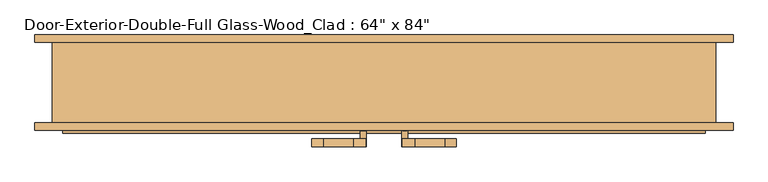
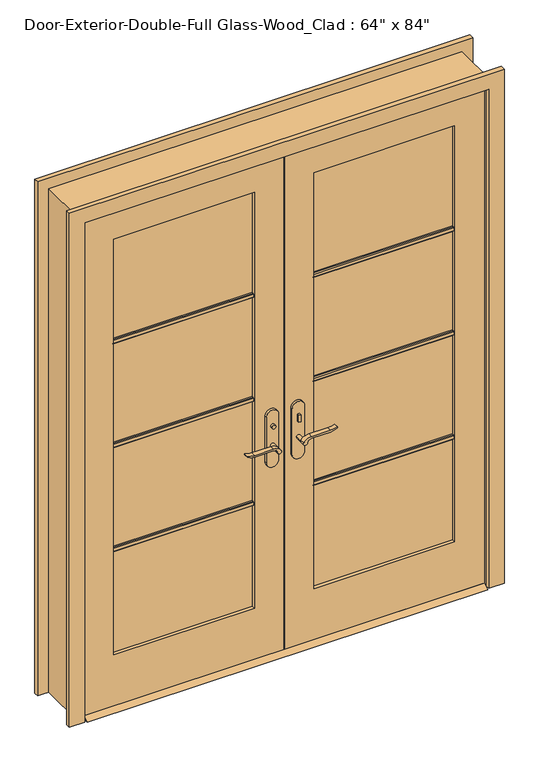
"""IFC4 building model written with IfcOpenShell, lengths in millimetres: door geometry."""

from ifc_helpers import new_model, si_unit, point, frame, frame_2d, origin, place, context, project, spatial, polyline, circle_curve, trimmed, segment, composite_curve, outline, extrude, faceted_brep, source, transform, mapped, element, save


def door_d93d7eea(model_context):
    return source(origin(), model_context, "Body", "SolidModel", [
        extrude(outline(polyline([(-63.5, 12.7), (-38.1, 0.0), (-123.825, 0.0), (-98.425, 12.7), (-63.5, 12.7)])), frame((-812.8, 0.0, 0.0), z_axis=(1.0, 0.0, 0.0), x_axis=(0.0, 1.0, 0.0)), (0.0, 0.0, 1.0), 1625.6),
        extrude(outline(polyline([(-47.4019111, -43.5), (-47.4019111, -53.5), (-57.4019111, -53.5), (-57.4019111, -43.5), (-47.4019111, -43.5)])), frame((0.0, 0.0, 981.9), z_axis=(0.0, 0.0, 1.0), x_axis=(1.0, 0.0, 0.0)), (0.0, 0.0, 1.0), 30.0),
        extrude(outline(composite_curve([segment(trimmed(circle_curve(frame_2d((996.9, -52.4019111)), 8.0), [point((996.9, -60.4019111))], [point((996.9, -44.4019111))], False, "CARTESIAN"), True, "CONTINUOUS"), segment(trimmed(circle_curve(frame_2d((996.9, -52.4019111)), 8.0), [point((996.9, -44.4019111))], [point((996.9, -60.4019111))], False, "CARTESIAN"), True, "CONTINUOUS")], self_intersect=False)), frame((0.0, -118.425, 0.0), z_axis=(0.0, 1.0, 0.0), x_axis=(0.0, 0.0, 1.0)), (0.0, 0.0, 1.0), 10.0),
        extrude(outline(composite_curve([segment(trimmed(circle_curve(frame_2d((897.1555521, -76.0694241)), 37.2832219), [point((919.0523287, -45.8937749))], [point((934.4, -77.7693445))], False, "CARTESIAN"), True, "CONTINUOUS"), segment(polyline([(934.4, -77.7693445), (934.4, -154.045502)]), True, "CONTINUOUS"), segment(trimmed(circle_curve(frame_2d((1017.6850638, -153.9791202)), 83.2850902), [point((934.4, -154.045502))], [point((939.4, -182.4019111))], True, "CARTESIAN"), True, "CONTINUOUS"), segment(polyline([(939.4, -182.4019111), (936.6135558, -182.4019111)]), True, "CONTINUOUS"), segment(trimmed(circle_curve(frame_2d((986.6709207, -150.4622499)), 59.3791355), [point((936.6135558, -182.4019111))], [point((927.4, -154.045502))], False, "CARTESIAN"), True, "CONTINUOUS"), segment(polyline([(927.4, -154.045502), (927.4, -77.7881013)]), True, "CONTINUOUS"), segment(trimmed(circle_curve(frame_2d((909.2738613, -77.7881013)), 18.1261387), [point((927.4, -77.7881013))], [point((914.4, -60.4019111))], True, "CARTESIAN"), True, "CONTINUOUS"), segment(trimmed(circle_curve(frame_2d((914.4, -52.4019111)), 8.0), [point((914.4, -60.4019111))], [point((919.0523287, -45.8937749))], False, "CARTESIAN"), True, "CONTINUOUS")], self_intersect=False)), frame((0.0, -23.5, 0.0), z_axis=(0.0, 1.0, 0.0), x_axis=(0.0, 0.0, 1.0)), (0.0, 0.0, 1.0), 20.0),
        extrude(outline(composite_curve([segment(trimmed(circle_curve(frame_2d((914.4, -52.4019111)), 8.0), [point((914.3999903, -60.4019111))], [point((919.0523287, -45.8937749))], False, "CARTESIAN"), True, "CONTINUOUS"), segment(trimmed(circle_curve(frame_2d((897.1555521, -76.0694241)), 37.2832219), [point((919.0523287, -45.8937749))], [point((934.4, -77.7693445))], False, "CARTESIAN"), True, "CONTINUOUS"), segment(polyline([(934.4, -77.7693445), (934.4, -154.045502)]), True, "CONTINUOUS"), segment(trimmed(circle_curve(frame_2d((1017.6850638, -153.9791202)), 83.2850902), [point((934.4, -154.045502))], [point((939.4, -182.4019111))], True, "CARTESIAN"), True, "CONTINUOUS"), segment(polyline([(939.4, -182.4019111), (936.6135558, -182.4019111)]), True, "CONTINUOUS"), segment(trimmed(circle_curve(frame_2d((986.6709207, -150.4622499)), 59.3791355), [point((936.6135558, -182.4019111))], [point((927.4, -154.045502))], False, "CARTESIAN"), True, "CONTINUOUS"), segment(polyline([(927.4, -154.045502), (927.4, -77.788099)]), True, "CONTINUOUS"), segment(trimmed(circle_curve(frame_2d((909.2738682, -77.788099)), 18.1261318), [point((927.4, -77.788099))], [point((914.3999903, -60.4019111))], True, "CARTESIAN"), True, "CONTINUOUS")], self_intersect=False)), frame((0.0, -158.425, 0.0), z_axis=(0.0, 1.0, 0.0), x_axis=(0.0, 0.0, 1.0)), (0.0, 0.0, 1.0), 20.0),
        extrude(outline(composite_curve([segment(trimmed(circle_curve(frame_2d((914.4, -52.4019111)), 8.0), [point((914.4, -60.4019111))], [point((914.4, -44.4019111))], False, "CARTESIAN"), True, "CONTINUOUS"), segment(trimmed(circle_curve(frame_2d((914.4, -52.4019111)), 8.0), [point((914.4, -44.4019111))], [point((914.4, -60.4019111))], False, "CARTESIAN"), True, "CONTINUOUS")], self_intersect=False)), frame((0.0, -53.5, 0.0), z_axis=(0.0, 1.0, 0.0), x_axis=(0.0, 0.0, 1.0)), (0.0, 0.0, 1.0), 30.0),
        extrude(outline(composite_curve([segment(trimmed(circle_curve(frame_2d((914.4, -52.4019111)), 8.0), [point((914.4, -60.4019111))], [point((914.4, -44.4019111))], False, "CARTESIAN"), True, "CONTINUOUS"), segment(trimmed(circle_curve(frame_2d((914.4, -52.4019111)), 8.0), [point((914.4, -44.4019111))], [point((914.4, -60.4019111))], False, "CARTESIAN"), True, "CONTINUOUS")], self_intersect=False)), frame((0.0, -138.425, 0.0), z_axis=(0.0, 1.0, 0.0), x_axis=(0.0, 0.0, 1.0)), (0.0, 0.0, 1.0), 30.0),
        extrude(outline(composite_curve([segment(polyline([(844.4, -27.4019111), (1039.4, -27.4019111)]), True, "CONTINUOUS"), segment(trimmed(circle_curve(frame_2d((1039.4, -52.4019111)), 25.0), [point((1039.4, -27.4019111))], [point((1039.4, -77.4019111))], False, "CARTESIAN"), True, "CONTINUOUS"), segment(polyline([(1039.4, -77.4019111), (844.4, -77.4019111)]), True, "CONTINUOUS"), segment(trimmed(circle_curve(frame_2d((844.4, -52.4019111)), 25.0), [point((844.4, -77.4019111))], [point((844.4, -27.4019111))], False, "CARTESIAN"), True, "CONTINUOUS")], self_intersect=False)), frame((0.0, -63.5, 0.0), z_axis=(0.0, 1.0, 0.0), x_axis=(0.0, 0.0, 1.0)), (0.0, 0.0, 1.0), 10.0),
        extrude(outline(composite_curve([segment(polyline([(844.4, -27.4019111), (1039.4, -27.4019111)]), True, "CONTINUOUS"), segment(trimmed(circle_curve(frame_2d((1039.4, -52.4019111)), 25.0), [point((1039.4, -27.4019111))], [point((1039.4, -77.4019111))], False, "CARTESIAN"), True, "CONTINUOUS"), segment(polyline([(1039.4, -77.4019111), (844.4, -77.4019111)]), True, "CONTINUOUS"), segment(trimmed(circle_curve(frame_2d((844.4, -52.4019111)), 25.0), [point((844.4, -77.4019111))], [point((844.4, -27.4019111))], False, "CARTESIAN"), True, "CONTINUOUS")], self_intersect=False)), frame((0.0, -108.425, 0.0), z_axis=(0.0, 1.0, 0.0), x_axis=(0.0, 0.0, 1.0)), (0.0, 0.0, 1.0), 10.0),
        extrude(outline(polyline([(47.3875, -118.425), (47.3875, -108.425), (57.3875, -108.425), (57.3875, -118.425), (47.3875, -118.425)])), frame((0.0, 0.0, 981.9), z_axis=(0.0, 0.0, 1.0), x_axis=(1.0, 0.0, 0.0)), (0.0, 0.0, 1.0), 30.0),
        extrude(outline(composite_curve([segment(trimmed(circle_curve(frame_2d((996.9, 52.3875)), 8.0), [point((996.9, 60.3875))], [point((996.9, 44.3875))], False, "CARTESIAN"), True, "CONTINUOUS"), segment(trimmed(circle_curve(frame_2d((996.9, 52.3875)), 8.0), [point((996.9, 44.3875))], [point((996.9, 60.3875))], False, "CARTESIAN"), True, "CONTINUOUS")], self_intersect=False)), frame((0.0, -53.5, 0.0), z_axis=(0.0, 1.0, 0.0), x_axis=(0.0, 0.0, 1.0)), (0.0, 0.0, 1.0), 10.0),
        extrude(outline(composite_curve([segment(trimmed(circle_curve(frame_2d((914.4, 52.3875)), 8.0), [point((919.0523287, 45.8793637))], [point((914.4, 60.3875))], False, "CARTESIAN"), True, "CONTINUOUS"), segment(trimmed(circle_curve(frame_2d((909.2738613, 77.7736901)), 18.1261387), [point((914.4, 60.3875))], [point((927.4, 77.7736901))], True, "CARTESIAN"), True, "CONTINUOUS"), segment(polyline([(927.4, 77.7736901), (927.4, 154.0310909)]), True, "CONTINUOUS"), segment(trimmed(circle_curve(frame_2d((986.6709207, 150.4478388)), 59.3791355), [point((927.4, 154.0310909))], [point((936.6135558, 182.3875))], False, "CARTESIAN"), True, "CONTINUOUS"), segment(polyline([(936.6135558, 182.3875), (939.4, 182.3875)]), True, "CONTINUOUS"), segment(trimmed(circle_curve(frame_2d((1017.6850638, 153.9647091)), 83.2850902), [point((939.4, 182.3875))], [point((934.4, 154.0310909))], True, "CARTESIAN"), True, "CONTINUOUS"), segment(polyline([(934.4, 154.0310909), (934.4, 77.7549333)]), True, "CONTINUOUS"), segment(trimmed(circle_curve(frame_2d((897.1555521, 76.0550129)), 37.2832219), [point((934.4, 77.7549333))], [point((919.0523287, 45.8793637))], False, "CARTESIAN"), True, "CONTINUOUS")], self_intersect=False)), frame((0.0, -158.425, 0.0), z_axis=(0.0, 1.0, 0.0), x_axis=(0.0, 0.0, 1.0)), (0.0, 0.0, 1.0), 20.0),
        extrude(outline(composite_curve([segment(trimmed(circle_curve(frame_2d((909.2738682, 77.7736878)), 18.1261318), [point((914.3999903, 60.3875))], [point((927.4, 77.7736878))], True, "CARTESIAN"), True, "CONTINUOUS"), segment(polyline([(927.4, 77.7736878), (927.4, 154.0310909)]), True, "CONTINUOUS"), segment(trimmed(circle_curve(frame_2d((986.6709207, 150.4478388)), 59.3791355), [point((927.4, 154.0310909))], [point((936.6135558, 182.3875))], False, "CARTESIAN"), True, "CONTINUOUS"), segment(polyline([(936.6135558, 182.3875), (939.4, 182.3875)]), True, "CONTINUOUS"), segment(trimmed(circle_curve(frame_2d((1017.6850638, 153.9647091)), 83.2850902), [point((939.4, 182.3875))], [point((934.4, 154.0310909))], True, "CARTESIAN"), True, "CONTINUOUS"), segment(polyline([(934.4, 154.0310909), (934.4, 77.7549333)]), True, "CONTINUOUS"), segment(trimmed(circle_curve(frame_2d((897.1555521, 76.0550129)), 37.2832219), [point((934.4, 77.7549333))], [point((919.0523287, 45.8793637))], False, "CARTESIAN"), True, "CONTINUOUS"), segment(trimmed(circle_curve(frame_2d((914.4, 52.3875)), 8.0), [point((919.0523287, 45.8793637))], [point((914.3999903, 60.3875))], False, "CARTESIAN"), True, "CONTINUOUS")], self_intersect=False)), frame((0.0, -23.5, 0.0), z_axis=(0.0, 1.0, 0.0), x_axis=(0.0, 0.0, 1.0)), (0.0, 0.0, 1.0), 20.0),
        extrude(outline(composite_curve([segment(trimmed(circle_curve(frame_2d((914.4, 52.3875)), 8.0), [point((914.4, 60.3875))], [point((914.4, 44.3875))], False, "CARTESIAN"), True, "CONTINUOUS"), segment(trimmed(circle_curve(frame_2d((914.4, 52.3875)), 8.0), [point((914.4, 44.3875))], [point((914.4, 60.3875))], False, "CARTESIAN"), True, "CONTINUOUS")], self_intersect=False)), frame((0.0, -138.425, 0.0), z_axis=(0.0, 1.0, 0.0), x_axis=(0.0, 0.0, 1.0)), (0.0, 0.0, 1.0), 30.0),
        extrude(outline(composite_curve([segment(trimmed(circle_curve(frame_2d((914.4, 52.3875)), 8.0), [point((914.4, 60.3875))], [point((914.4, 44.3875))], False, "CARTESIAN"), True, "CONTINUOUS"), segment(trimmed(circle_curve(frame_2d((914.4, 52.3875)), 8.0), [point((914.4, 44.3875))], [point((914.4, 60.3875))], False, "CARTESIAN"), True, "CONTINUOUS")], self_intersect=False)), frame((0.0, -53.5, 0.0), z_axis=(0.0, 1.0, 0.0), x_axis=(0.0, 0.0, 1.0)), (0.0, 0.0, 1.0), 30.0),
        extrude(outline(composite_curve([segment(trimmed(circle_curve(frame_2d((844.4, 52.3875)), 25.0), [point((844.4, 27.3875))], [point((844.4, 77.3875))], False, "CARTESIAN"), True, "CONTINUOUS"), segment(polyline([(844.4, 77.3875), (1039.4, 77.3875)]), True, "CONTINUOUS"), segment(trimmed(circle_curve(frame_2d((1039.4, 52.3875)), 25.0), [point((1039.4, 77.3875))], [point((1039.4, 27.3875))], False, "CARTESIAN"), True, "CONTINUOUS"), segment(polyline([(1039.4, 27.3875), (844.4, 27.3875)]), True, "CONTINUOUS")], self_intersect=False)), frame((0.0, -108.425, 0.0), z_axis=(0.0, 1.0, 0.0), x_axis=(0.0, 0.0, 1.0)), (0.0, 0.0, 1.0), 10.0),
        extrude(outline(composite_curve([segment(trimmed(circle_curve(frame_2d((844.4, 52.3875)), 25.0), [point((844.4, 27.3875))], [point((844.4, 77.3875))], False, "CARTESIAN"), True, "CONTINUOUS"), segment(polyline([(844.4, 77.3875), (1039.4, 77.3875)]), True, "CONTINUOUS"), segment(trimmed(circle_curve(frame_2d((1039.4, 52.3875)), 25.0), [point((1039.4, 77.3875))], [point((1039.4, 27.3875))], False, "CARTESIAN"), True, "CONTINUOUS"), segment(polyline([(1039.4, 27.3875), (844.4, 27.3875)]), True, "CONTINUOUS")], self_intersect=False)), frame((0.0, -63.5, 0.0), z_axis=(0.0, 1.0, 0.0), x_axis=(0.0, 0.0, 1.0)), (0.0, 0.0, 1.0), 10.0),
        extrude(outline(polyline([(-77.47, 1578.371875), (-71.12, 1578.371875), (-67.945, 1575.196875), (-67.945, 1562.496875), (-71.12, 1559.321875), (-77.47, 1559.321875), (-77.47, 1578.371875)])), frame((120.65, 0.0, 0.0), z_axis=(1.0, 0.0, 0.0), x_axis=(0.0, 1.0, 0.0)), (0.0, 0.0, 1.0), 571.5),
        extrude(outline(polyline([(-77.47, 1132.68125), (-71.12, 1132.68125), (-67.945, 1129.50625), (-67.945, 1116.80625), (-71.12, 1113.63125), (-77.47, 1113.63125), (-77.47, 1132.68125)])), frame((120.65, 0.0, 0.0), z_axis=(1.0, 0.0, 0.0), x_axis=(0.0, 1.0, 0.0)), (0.0, 0.0, 1.0), 571.5),
        extrude(outline(polyline([(-77.47, 686.990625), (-71.12, 686.990625), (-67.945, 683.815625), (-67.945, 671.115625), (-71.12, 667.940625), (-77.47, 667.940625), (-77.47, 686.990625)])), frame((120.65, 0.0, 0.0), z_axis=(1.0, 0.0, 0.0), x_axis=(0.0, 1.0, 0.0)), (0.0, 0.0, 1.0), 571.5),
        extrude(outline(polyline([(-84.455, 1578.371875), (-84.455, 1559.321875), (-90.805, 1559.321875), (-93.98, 1562.496875), (-93.98, 1575.196875), (-90.805, 1578.371875), (-84.455, 1578.371875)])), frame((-692.15, 0.0, 0.0), z_axis=(1.0, 0.0, 0.0), x_axis=(0.0, 1.0, 0.0)), (0.0, 0.0, 1.0), 571.5),
        extrude(outline(polyline([(-84.455, 1132.68125), (-84.455, 1113.63125), (-90.805, 1113.63125), (-93.98, 1116.80625), (-93.98, 1129.50625), (-90.805, 1132.68125), (-84.455, 1132.68125)])), frame((-692.15, 0.0, 0.0), z_axis=(1.0, 0.0, 0.0), x_axis=(0.0, 1.0, 0.0)), (0.0, 0.0, 1.0), 571.5),
        extrude(outline(polyline([(-84.455, 686.990625), (-84.455, 667.940625), (-90.805, 667.940625), (-93.98, 671.115625), (-93.98, 683.815625), (-90.805, 686.990625), (-84.455, 686.990625)])), frame((-692.15, 0.0, 0.0), z_axis=(1.0, 0.0, 0.0), x_axis=(0.0, 1.0, 0.0)), (0.0, 0.0, 1.0), 571.5),
        extrude(outline(polyline([(-84.455, 1578.371875), (-84.455, 1559.321875), (-90.805, 1559.321875), (-93.98, 1562.496875), (-93.98, 1575.196875), (-90.805, 1578.371875), (-84.455, 1578.371875)])), frame((120.65, 0.0, 0.0), z_axis=(1.0, 0.0, 0.0), x_axis=(0.0, 1.0, 0.0)), (0.0, 0.0, 1.0), 571.5),
        extrude(outline(polyline([(-84.455, 1132.68125), (-84.455, 1113.63125), (-90.805, 1113.63125), (-93.98, 1116.80625), (-93.98, 1129.50625), (-90.805, 1132.68125), (-84.455, 1132.68125)])), frame((120.65, 0.0, 0.0), z_axis=(1.0, 0.0, 0.0), x_axis=(0.0, 1.0, 0.0)), (0.0, 0.0, 1.0), 571.5),
        extrude(outline(polyline([(-84.455, 686.990625), (-84.455, 667.940625), (-90.805, 667.940625), (-93.98, 671.115625), (-93.98, 683.815625), (-90.805, 686.990625), (-84.455, 686.990625)])), frame((120.65, 0.0, 0.0), z_axis=(1.0, 0.0, 0.0), x_axis=(0.0, 1.0, 0.0)), (0.0, 0.0, 1.0), 571.5),
        extrude(outline(polyline([(-77.47, 1578.371875), (-71.12, 1578.371875), (-67.945, 1575.196875), (-67.945, 1562.496875), (-71.12, 1559.321875), (-77.47, 1559.321875), (-77.47, 1578.371875)])), frame((-692.15, 0.0, 0.0), z_axis=(1.0, 0.0, 0.0), x_axis=(0.0, 1.0, 0.0)), (0.0, 0.0, 1.0), 571.5),
        extrude(outline(polyline([(-77.47, 1132.68125), (-71.12, 1132.68125), (-67.945, 1129.50625), (-67.945, 1116.80625), (-71.12, 1113.63125), (-77.47, 1113.63125), (-77.47, 1132.68125)])), frame((-692.15, 0.0, 0.0), z_axis=(1.0, 0.0, 0.0), x_axis=(0.0, 1.0, 0.0)), (0.0, 0.0, 1.0), 571.5),
        extrude(outline(polyline([(-77.47, 686.990625), (-71.12, 686.990625), (-67.945, 683.815625), (-67.945, 671.115625), (-71.12, 667.940625), (-77.47, 667.940625), (-77.47, 686.990625)])), frame((-692.15, 0.0, 0.0), z_axis=(1.0, 0.0, 0.0), x_axis=(0.0, 1.0, 0.0)), (0.0, 0.0, 1.0), 571.5),
        extrude(outline(polyline([(0.0, 882.65), (2203.45, 882.65), (2203.45, -882.65), (0.0, -882.65), (0.0, -819.15), (2139.95, -819.15), (2139.95, 819.15), (0.0, 819.15), (0.0, 882.65)])), frame((0.0, -117.475, 0.0), z_axis=(0.0, 1.0, 0.0), x_axis=(0.0, 0.0, 1.0)), (0.0, 0.0, 1.0), 19.05),
        extrude(outline(polyline([(0.0, 882.65), (2203.45, 882.65), (2203.45, -882.65), (0.0, -882.65), (0.0, -819.15), (2139.95, -819.15), (2139.95, 819.15), (0.0, 819.15), (0.0, 882.65)])), frame((0.0, 104.775, 0.0), z_axis=(0.0, 1.0, 0.0), x_axis=(0.0, 0.0, 1.0)), (0.0, 0.0, 1.0), 19.05),
        extrude(outline(polyline([(2133.6, 812.8), (2133.6, 1.5875), (12.7, 1.5875), (12.7, 812.8), (2133.6, 812.8)]), holes=[polyline([(2014.5375, 120.65), (2014.5375, 692.15), (231.775, 692.15), (231.775, 120.65), (2014.5375, 120.65)])]), frame((0.0, -98.425, 0.0), z_axis=(0.0, 1.0, 0.0), x_axis=(0.0, 0.0, 1.0)), (0.0, 0.0, 1.0), 34.925),
        extrude(outline(polyline([(12.7, -812.8), (12.7, -1.6019111), (2133.6, -1.6019111), (2133.6, -812.8), (12.7, -812.8)]), holes=[polyline([(231.775, -692.15), (2014.5375, -692.15), (2014.5375, -120.65), (231.775, -120.65), (231.775, -692.15)])]), frame((0.0, -98.425, 0.0), z_axis=(0.0, 1.0, 0.0), x_axis=(0.0, 0.0, 1.0)), (0.0, 0.0, 1.0), 34.925),
        faceted_brep([(838.2, -98.425, 0.0), (812.8, -98.425, 0.0), (812.8, -63.5, 0.0), (800.1, -63.5, 0.0), (800.1, -28.575, 0.0), (812.8, -28.575, 0.0), (812.8, 104.775, 0.0), (838.2, 104.775, 0.0), (838.2, 104.775, 2159.0), (838.2, -98.425, 2159.0), (812.8, 104.775, 2133.6), (-812.8, 104.775, 2133.6), (-812.8, 104.775, 0.0), (-838.2, 104.775, 0.0), (-838.2, 104.775, 2159.0), (812.8, -28.575, 2133.6), (800.1, -28.575, 2120.9), (-800.1, -28.575, 2120.9), (-800.1, -28.575, 0.0), (-812.8, -28.575, 0.0), (-812.8, -28.575, 2133.6), (800.1, -63.5, 2120.9), (812.8, -63.5, 2133.6), (1.5875, -63.5, 2133.6), (-1.6019111, -63.5, 2133.6), (-812.8, -63.5, 2133.6), (-812.8, -63.5, 0.0), (-800.1, -63.5, 0.0), (-800.1, -63.5, 2120.9), (-1.6019111, -63.5, 2120.9), (1.5875, -63.5, 2120.9), (812.8, -98.425, 2133.6), (-838.2, -98.425, 2159.0), (-838.2, -98.425, 0.0), (-812.8, -98.425, 0.0), (-812.8, -98.425, 2133.6), (-1.6019111, -98.425, 2133.6), (1.5875, -98.425, 2133.6)], [[[0, 1, 2, 3, 4, 5, 6, 7]], [[7, 8, 9, 0]], [[6, 10, 11, 12, 13, 14, 8, 7]], [[5, 15, 10, 6]], [[4, 16, 17, 18, 19, 20, 15, 5]], [[3, 21, 16, 4]], [[2, 22, 23, 24, 25, 26, 27, 28, 29, 30, 21, 3]], [[1, 31, 22, 2]], [[0, 9, 32, 33, 34, 35, 36, 37, 31, 1]], [[8, 14, 32, 9]], [[10, 15, 20, 11]], [[16, 21, 30, 29, 28, 17]], [[31, 37, 36, 35, 25, 24, 23, 22]], [[12, 19, 18, 27, 26, 34, 33, 13]], [[13, 33, 32, 14]], [[11, 20, 19, 12]], [[17, 28, 27, 18]], [[25, 35, 34, 26]]]),
        extrude(outline(polyline([(692.15, -77.47), (692.15, -84.455), (120.65, -84.455), (120.65, -77.47), (692.15, -77.47)])), frame((0.0, 0.0, 231.775), z_axis=(0.0, 0.0, 1.0), x_axis=(1.0, 0.0, 0.0)), (0.0, 0.0, 1.0), 1782.7625),
        extrude(outline(polyline([(-120.65, -77.47), (-120.65, -84.455), (-692.15, -84.455), (-692.15, -77.47), (-120.65, -77.47)])), frame((0.0, 0.0, 231.775), z_axis=(0.0, 0.0, 1.0), x_axis=(1.0, 0.0, 0.0)), (0.0, 0.0, 1.0), 1782.7625),
    ])


if __name__ == "__main__":
    model = new_model("IFC4")
    model_context = context("Model", 3, world=origin())
    ifc_project = project(units=[si_unit("LENGTHUNIT", "METRE", prefix="MILLI")], contexts=[model_context])
    site = spatial("IfcSite", under=ifc_project)
    building = spatial("IfcBuilding", under=site)
    placement = place(None, origin())
    door_shape = door_d93d7eea(model_context)
    element("IfcDoor", 1, ObjectType="Door-Exterior-Double-Full Glass-Wood_Clad : 64\" x 84\"", at=placement, inside=building, context=model_context, shape_type="MappedRepresentation", body=[
        mapped(door_shape, transform((0.0, 0.0, 0.0), x_axis=(1.0, 0.0, 0.0), y_axis=(0.0, 1.0, 0.0), z_axis=(0.0, 0.0, 1.0))),
    ])
    save(model, "model.ifc")

# Revit data of these elements
# Type "Door-Exterior-Double-Full Glass-Wood_Clad : 64\" x 84\""
#   Type Mark = "9"
#   Assembly Code = "B2030100"
#   Analytic Construction = "French door, wood frame with double glass"
#   Top Rail = 0' - 4 11/16"
#   Threshold Offset [instance default] = 0' - 0 1/2"
#   Thickness = 0' - 1 3/8"
#   Thermal Resistance (R) = 1.9158 (h·ft²·°F)/BTU
#   Swing Angle [instance default] = 90.00°
#   Stiles = 0' - 4 3/4"
#   Rough Width = 5' - 6"
#   Rough Height = 7' - 1"
#   Panel Width = 2' - 8"
#   Door Offset [instance default] = 0' - 0"
#   Height = 7' - 0"
#   Width = 5' - 4"
#   Heat Transfer Coefficient (U) = 0.5220 BTU/(h·ft²·°F)
#   Bottom Rail = 0' - 9 1/8"
#   Exterior Trim [instance default] = yes
#   Threshold [instance default] = yes
#   Show Grill [instance default] = yes
#   Function = 1
#   Trim Material = Cherry
#   Threshold Material = Cherry
#   Panel Material = Cherry
#   Glazing = Glass
#   Frame Material = Cherry
#   Door Handle Material = Aluminum
#   Visual Light Transmittance = 0
#   Solar Heat Gain Coefficient = 0
#   Wall Closure = (empty or 0)
#   Construction Type = (empty or 0)
# Element 1 (IfcDoor, "Door-Exterior-Double-Full Glass-Wood_Clad : 64\" x 84\"")
#   Materials on its faces: "Cherry", "Aluminum", "Glass"
# Materials
#   "Cherry": class "Wood", colour RGB 226 177 128, transparency 0, Description = "Prunus Serotina", Cost = 0
#   "Glass": class "Glass", colour RGB 0 128 192, transparency 0.75, Description = "Soda Lime Glass", Cost = 0
#   "Aluminum": class "Metal", colour RGB 247 247 247, transparency 0, Description = "Aluminum 6061", Cost = 0
